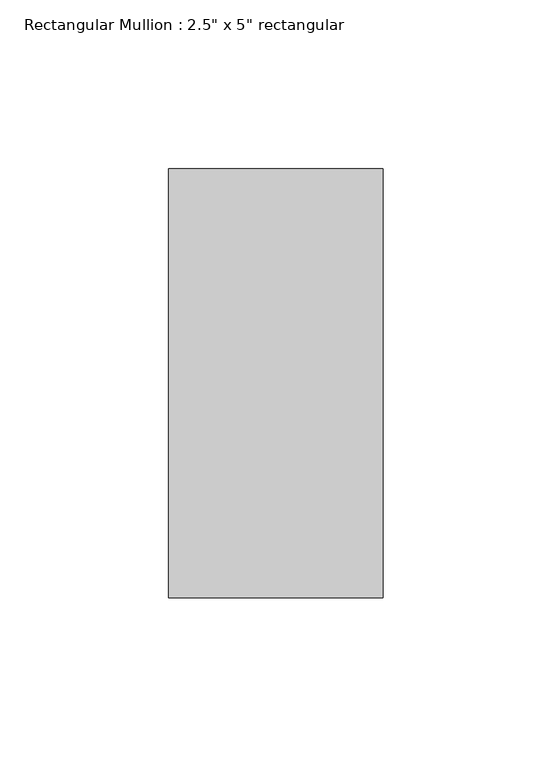
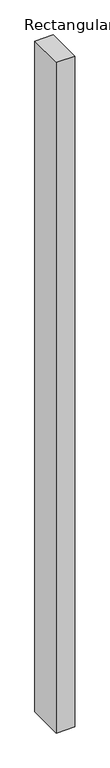
"""IFC4 building model written with IfcOpenShell, lengths in millimetres: member geometry."""

from ifc_helpers import new_model, si_unit, frame, origin, place, context, project, spatial, polyline, outline, extrude, source, transform, mapped, element, save


def member_f0fea5a5(model_context):
    return source(origin(), model_context, "Body", "SweptSolid", [
        extrude(outline(polyline([(31.75, 63.5), (31.75, -63.5), (-31.75, -63.5), (-31.75, 63.5), (31.75, 63.5)])), frame((0.0, 0.0, -2438.4), z_axis=(0.0, 0.0, 1.0), x_axis=(1.0, 0.0, 0.0)), (0.0, 0.0, 1.0), 2438.4),
    ])


if __name__ == "__main__":
    model = new_model("IFC4")
    model_context = context("Model", 3, world=origin())
    ifc_project = project(units=[si_unit("LENGTHUNIT", "METRE", prefix="MILLI")], contexts=[model_context])
    site = spatial("IfcSite", under=ifc_project)
    building = spatial("IfcBuilding", under=site)
    placement = place(None, origin())
    member_shape = member_f0fea5a5(model_context)
    element("IfcMember", 1, ObjectType="Rectangular Mullion : 2.5\" x 5\" rectangular", at=placement, inside=building, context=model_context, shape_type="MappedRepresentation", body=[
        mapped(member_shape, transform((0.0, 0.0, 0.0), x_axis=(1.0, 0.0, 0.0), y_axis=(0.0, 1.0, 0.0), z_axis=(0.0, 0.0, 1.0))),
    ])
    save(model, "model.ifc")

# Revit data of these elements
# Type "Rectangular Mullion : 2.5\" x 5\" rectangular"
#   built-in parameter 1007304 = 0.416667 (stored number, unit not read)
#   built-in parameter 1007301 = 0.104167 (stored number, unit not read)
#   built-in parameter 1007300 = 0.104167 (stored number, unit not read)
# Element 1 (IfcMember, "Rectangular Mullion : 2.5\" x 5\" rectangular")
#   Materials on its faces: "BLACK COLOUR"
# Materials
#   "BLACK COLOUR": class "Generic", colour RGB 120 120 120, transparency 0, Cost = 0
